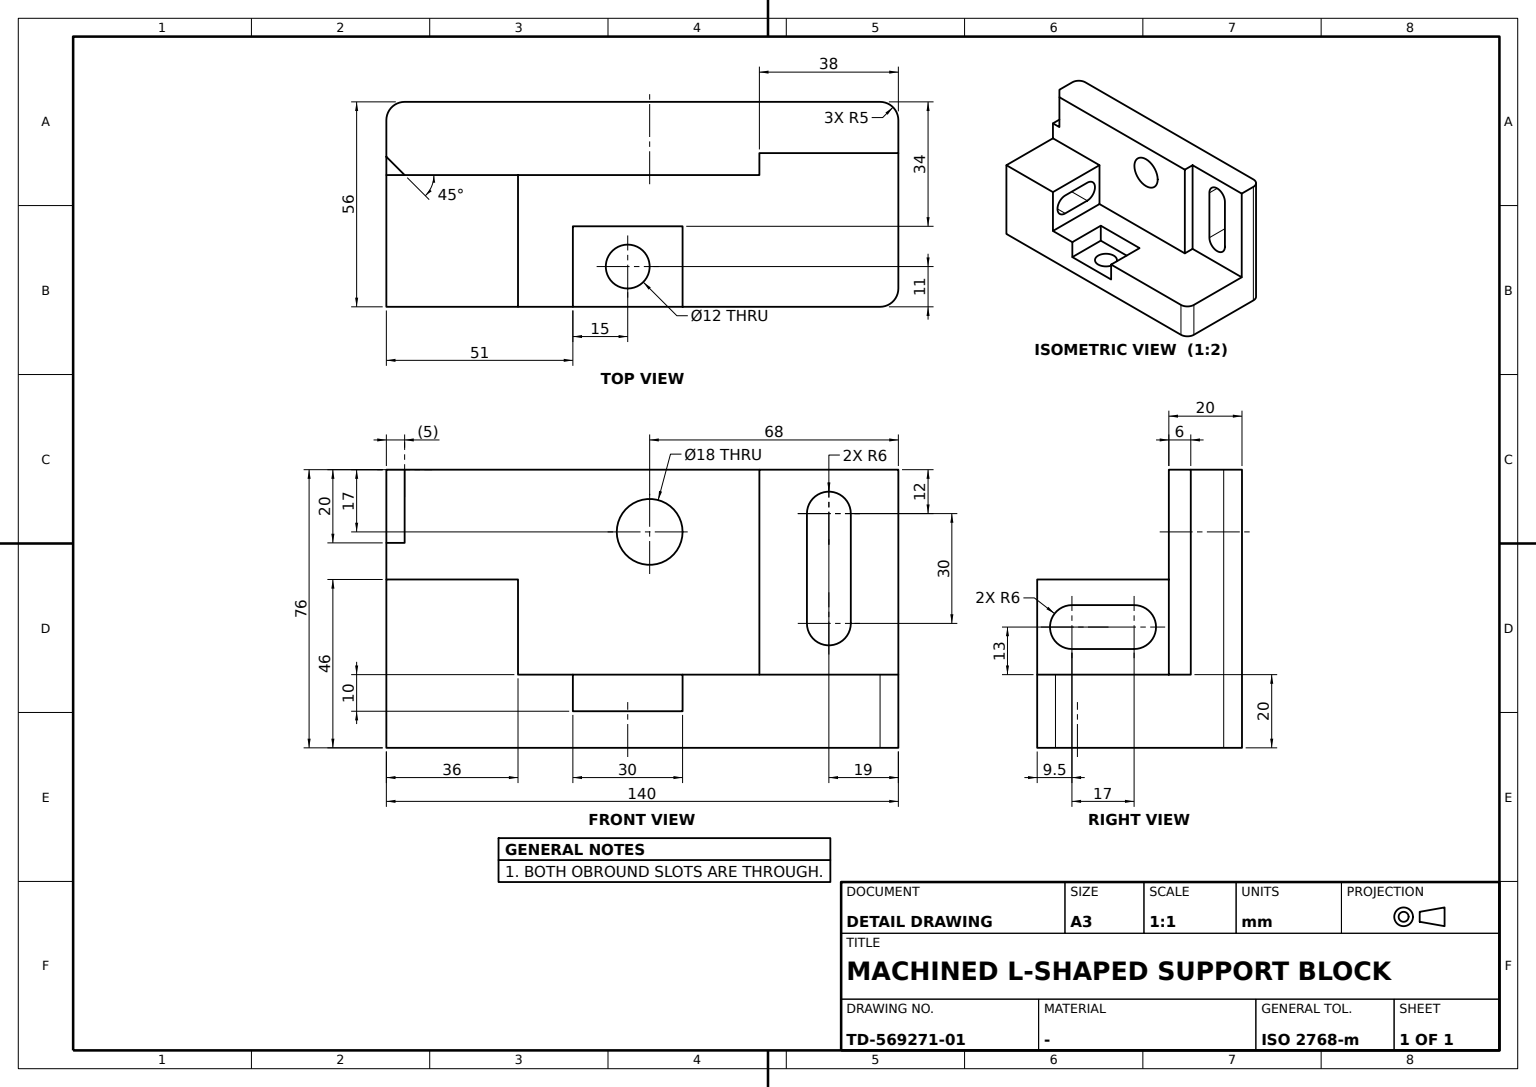
CATIA V5 part; units mm, degrees
sketch "Sketch1" plane through (0, 0, 0) normal (0, 1, 0) x (-1, 0, 0)
  line L0 (0, 0) -> (0, 76)
  point P0 (0, 76)
  line L1 (0, 76) -> (-20, 76)
  point P1 (0, 76)
  line L2 (0, 0) -> (-56, 0)
  line L3 (-56, 0) -> (-56, 20)
  line L4 (-20, 76) -> (-20, 20)
  line L5 (-56, 20) -> (-20, 20)
  dimension "length L0" = 76
  dimension "length L1" = 20
  dimension "length L2" = 56
  dimension "length L3" = 20
  constraint vertical L0 y-axis
  constraint vertical L3 y-axis
  constraint vertical L4 y-axis
  constraint horizontal L1 x-axis
  constraint horizontal L2 x-axis
  constraint horizontal L5 x-axis
  constraint coincidence P1 P0
extrude "Pad1" add sketch "Sketch1" along normal mid plane 140
sketch "Sketch2" plane through (20, 0, 0) normal (1, 0, 0) x (0, 1, 0)
  point P0 (51, 48)
  line L0 (70, 76) -> (70, 20)
  line L1 (70, 20) -> (32, 20)
  line L2 (32, 20) -> (32, 76)
  line L3 (32, 76) -> (70, 76)
  line L4 (70, 76) -> (70, 20) construction
  line L5 (-70, 20) -> (70, 20) construction
  line L6 (-70, 76) -> (70, 76) construction
  dimension "length L3" = 38
  constraint vertical L0 y-axis
  constraint vertical L2 y-axis
  constraint horizontal L1 x-axis
  constraint horizontal L3 x-axis
  constraint equidistance L0 L2 P0
  constraint equidistance L1 L3 P0
  constraint coincidence L0 L4
  constraint coincidence L1 L5
  constraint coincidence L3 L6
extrude "Pocket1" cut sketch "Sketch2" against normal blind 6
sketch "Sketch3" plane through (14, 0, 0) normal (1, 0, 0) x (0, 1, 0)
  point P0 (51, 49)
  line L0 (57, 64) -> (57, 34)
  line L1 (45, 34) -> (45, 64)
  point P1 (57, 34)
  point P2 (45, 34)
  line L2 (70, 20) -> (70, 76) construction
  arc A0 (45, 64) -> (57, 64) centre (51, 64) cw
  arc A1 (45, 34) -> (57, 34) centre (51, 34) ccw
  dimension "length L1" = 30
  dimension "distance P0 L2" = 19
  dimension "distance P1 P2" = 12
  constraint vertical L0 y-axis
  constraint vertical L1 y-axis
  constraint equidistance L0 L1 P0
  constraint tangency A0 L0
  constraint tangency A1 L0
extrude "Pocket2" cut sketch "Sketch3" against normal up to next
fillet "Fillet1" radius 5 1 edges at (56, 70, 10)
fillet "Fillet2" radius 5 1 edges at (0, 70, 38)
sketch "Sketch4" plane through (0, 0, 20) normal (0, 0, 1) x (1, 0, 0)
  point P0 (45, -4)
  line L0 (56, 11) -> (56, -19)
  line L1 (56, -19) -> (34, -19)
  line L2 (34, -19) -> (34, 11)
  line L3 (34, 11) -> (56, 11)
  line L4 (20, -70) -> (56, -70) construction
  line L5 (56, -70) -> (56, 70) construction
  dimension "distance L1 L4" = 51
  dimension "length L0" = 30
  dimension "length L3" = 22
  constraint vertical L0 y-axis
  constraint vertical L2 y-axis
  constraint horizontal L1 x-axis
  constraint horizontal L3 x-axis
  constraint equidistance L0 L2 P0
  constraint equidistance L1 L3 P0
  constraint coincidence L0 L5
extrude "Pocket3" cut sketch "Sketch4" against normal blind 10
sketch "Sketch5" plane through (0, 0, 10) normal (0, 0, 1) x (1, 0, 0)
  circle A0 centre (45, -4) radius 6
  point P0 (45, -4)
  line L0 (56, 11) -> (34, 11) construction
  line L1 (34, 11) -> (34, -19) construction
  dimension "radius A0" = 6
  dimension "distance P0 L0" = 15
  dimension "distance P0 L1" = 11
extrude "Pocket4" cut sketch "Sketch5" against normal blind 10
sketch "Sketch6" plane through (0, 0, 20) normal (0, 0, 1) x (1, 0, 0)
  point P0 (38, -52)
  line L0 (56, -34) -> (56, -70)
  line L1 (56, -70) -> (20, -70)
  line L2 (20, -70) -> (20, -34)
  line L3 (20, -34) -> (56, -34)
  line L4 (20, -70) -> (56, -70) construction
  line L5 (56, -70) -> (56, 70) construction
  dimension "length L1" = 36
  dimension "length L0" = 36
  constraint vertical L0 y-axis
  constraint vertical L2 y-axis
  constraint horizontal L1 x-axis
  constraint horizontal L3 x-axis
  constraint equidistance L0 L2 P0
  constraint equidistance L1 L3 P0
  constraint coincidence L1 L4
  constraint coincidence L0 L5
extrude "Pad2" add sketch "Sketch6" along normal blind 26
sketch "Sketch7" plane through (0, -34, 0) normal (0, 1, 0) x (-1, 0, 0)
  point P0 (-38, 33)
  line L0 (-29.5, 27) -> (-46.5, 27)
  line L1 (-46.5, 39) -> (-29.5, 39)
  point P1 (-29.5, 39)
  point P2 (-29.5, 27)
  line L2 (-56, 46) -> (-20, 46) construction
  line L3 (-20, 76) -> (-20, 20) construction
  arc A0 (-46.5, 39) -> (-46.5, 27) centre (-46.5, 33) ccw
  arc A1 (-29.5, 39) -> (-29.5, 27) centre (-29.5, 33) cw
  dimension "distance P0 L2" = 13
  dimension "length L0" = 17
  dimension "distance P0 L3" = 18
  dimension "distance P1 P2" = 12
  constraint horizontal L0 x-axis
  constraint horizontal L1 x-axis
  constraint equidistance L0 L1 P0
  constraint tangency A0 L0
  constraint tangency A1 L0
extrude "Pocket5" cut sketch "Sketch7" against normal up to next
fillet "Fillet3" radius 5 1 edges at (0, -70, 38)
chamfer "Chamfer1" distance 5 distance2 5 1 edges at (20, -70, 61)
sketch "Sketch8" plane through (20, 0, 0) normal (1, 0, 0) x (0, 1, 0)
  point P0 (-61.7562, 51)
  line L0 (-53.5124, 56) -> (-53.5124, 46)
  line L1 (-53.5124, 46) -> (-70, 46)
  line L2 (-70, 46) -> (-70, 56)
  line L3 (-70, 56) -> (-53.5124, 56)
  line L4 (-70, 46) -> (-34, 46) construction
  line L5 (-70, 76) -> (-70, 46) construction
  dimension "length L2" = 10
  constraint vertical L0 y-axis
  constraint vertical L2 y-axis
  constraint horizontal L1 x-axis
  constraint horizontal L3 x-axis
  constraint equidistance L0 L2 P0
  constraint equidistance L1 L3 P0
  constraint coincidence L1 L4
  constraint coincidence L2 L5
extrude "Pad3" add sketch "Sketch8" against normal blind 10
sketch "Sketch9" plane through (20, 0, 0) normal (1, 0, 0) x (0, 1, 0)
  circle A0 centre (2, 59) radius 9
  point P0 (2, 59)
  line L0 (32, 76) -> (32, 20) construction
  line L1 (-70, 76) -> (70, 76) construction
  dimension "distance P0 L0" = 30
  dimension "distance L1 P0" = 17
  dimension "radius A0" = 9
extrude "Pocket6" cut sketch "Sketch9" against normal up to next
